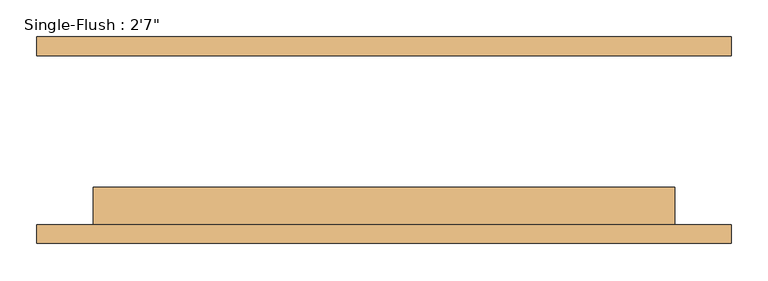
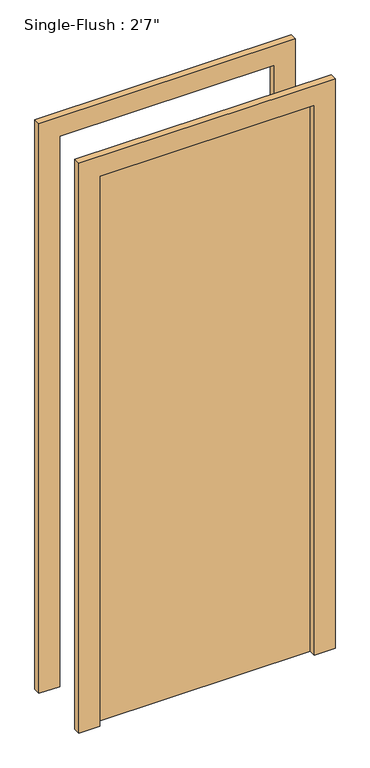
"""IFC4 building model written with IfcOpenShell, lengths in millimetres: door geometry."""

from ifc_helpers import new_model, si_unit, frame, origin, origin_with_axes, place, context, project, spatial, polyline, outline, extrude, source, transform, mapped, element, save


def door_486760f8(model_context):
    return source(origin(), model_context, "Body", "SweptSolid", [
        extrude(outline(polyline([(2209.8, -469.9), (0.0, -469.9), (0.0, -393.7), (2133.6, -393.7), (2133.6, 393.7), (0.0, 393.7), (0.0, 469.9), (2209.8, 469.9), (2209.8, -469.9)])), frame((0.0, -139.7, 0.0), z_axis=(0.0, 1.0, 0.0), x_axis=(0.0, 0.0, 1.0)), (0.0, 0.0, 1.0), 25.4),
        extrude(outline(polyline([(2209.8, 469.9), (2209.8, -469.9), (0.0, -469.9), (0.0, -393.7), (2133.6, -393.7), (2133.6, 393.7), (0.0, 393.7), (0.0, 469.9), (2209.8, 469.9)])), frame((0.0, 114.3, 0.0), z_axis=(0.0, 1.0, 0.0), x_axis=(0.0, 0.0, 1.0)), (0.0, 0.0, 1.0), 25.4),
        extrude(outline(polyline([(393.7, -63.5), (393.7, -114.3), (-393.7, -114.3), (-393.7, -63.5), (393.7, -63.5)])), origin_with_axes(), (0.0, 0.0, 1.0), 2133.6),
    ])


if __name__ == "__main__":
    model = new_model("IFC4")
    model_context = context("Model", 3, world=origin())
    ifc_project = project(units=[si_unit("LENGTHUNIT", "METRE", prefix="MILLI")], contexts=[model_context])
    site = spatial("IfcSite", under=ifc_project)
    building = spatial("IfcBuilding", under=site)
    placement = place(None, origin())
    door_shape = door_486760f8(model_context)
    element("IfcDoor", 1, ObjectType="Single-Flush : 2'7\"", at=placement, inside=building, context=model_context, shape_type="MappedRepresentation", body=[
        mapped(door_shape, transform((0.0, 0.0, 0.0), x_axis=(1.0, 0.0, 0.0), y_axis=(0.0, 1.0, 0.0), z_axis=(0.0, 0.0, 1.0))),
    ])
    save(model, "model.ifc")

# Revit data of these elements
# Type "Single-Flush : 2'7\""
#   Type Mark = "8"
#   Construction Type Id = "MDOOR"
#   Assembly Code = "C1020"
#   Analytic Construction = "Metal"
#   Thickness = 0' - 2"
#   Heat Transfer Coefficient (U) = 0.651978 BTU/(h·ft²·°F)
#   Height = 7' - 0"
#   Trim Projection Ext = 0' - 1"
#   Trim Projection Int = 0' - 1"
#   Trim Width = 0' - 3"
#   Width = 2' - 7"
#   Define Thermal Properties by = 1
#   Door Material = Door - Panel
#   Frame Material = Door - Frame
#   Visual Light Transmittance = 0
#   Solar Heat Gain Coefficient = 0
#   Function = (empty or 0)
#   Wall Closure = (empty or 0)
# Element 1 (IfcDoor, "Single-Flush : 2'7\"")
#   Materials on its faces: "Door - Frame", "Door - Panel"
# Materials
#   "Door - Panel": class "Wood", colour RGB 210 159 95, transparency 0
#   "Door - Frame": colour RGB 118 70 51, transparency 0
